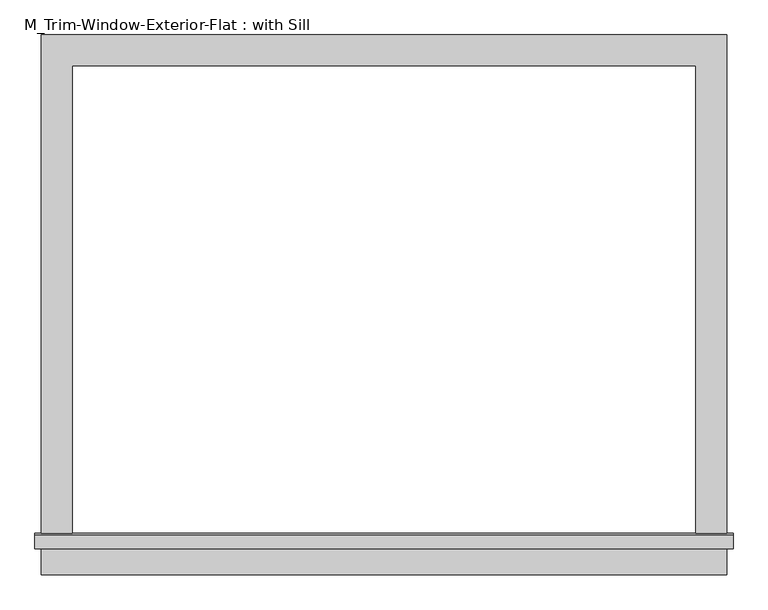
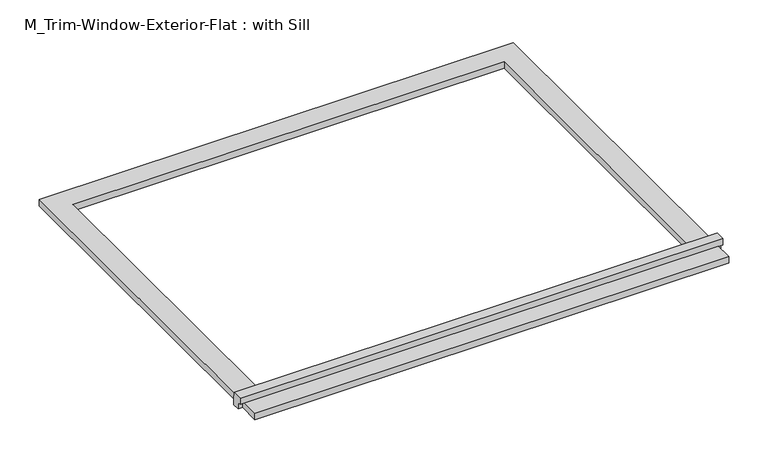
"""IFC4 building model written with IfcOpenShell, lengths in millimetres: proxy geometry, M_Trim-Window-Exterior-Flat : with Sill."""

from ifc_helpers import new_model, si_unit, frame, origin, origin_with_axes, place, context, project, spatial, polyline, outline, extrude, source, transform, mapped, element, save


def m_trim_window_exterior_flat_with_sill_6ae8fed8(model_context):
    return source(origin(), model_context, "Body", "SweptSolid", [
        extrude(outline(polyline([(669.6, -934.8323709), (669.6, -994.8323709), (-669.6, -994.8323709), (-669.6, -934.8323709), (669.6, -934.8323709)])), origin_with_axes(), (0.0, 0.0, 1.0), 19.05),
        extrude(outline(polyline([(-944.4, 38.1), (-916.8580645, 38.1), (-914.4, 19.05), (-914.4, 0.0), (-934.8323709, 0.0), (-934.8323709, 19.05), (-944.4, 19.05), (-944.4, 38.1)])), frame((-682.3, 0.0, 0.0), z_axis=(1.0, 0.0, 0.0), x_axis=(0.0, 1.0, 0.0)), (0.0, 0.0, 1.0), 1364.6),
        extrude(outline(polyline([(-669.6, 60.0), (669.6, 60.0), (669.6, -914.4), (609.6, -914.4), (609.6, 0.0), (-609.6, 0.0), (-609.6, -914.4), (-669.6, -914.4), (-669.6, 60.0)])), origin_with_axes(), (0.0, 0.0, 1.0), 19.05),
    ])


if __name__ == "__main__":
    model = new_model("IFC4")
    model_context = context("Model", 3, world=origin())
    ifc_project = project(units=[si_unit("LENGTHUNIT", "METRE", prefix="MILLI")], contexts=[model_context])
    site = spatial("IfcSite", under=ifc_project)
    building = spatial("IfcBuilding", under=site)
    placement = place(None, origin())
    m_trim_window_exterior_flat_with_sill_shape = m_trim_window_exterior_flat_with_sill_6ae8fed8(model_context)
    element("IfcBuildingElementProxy", 1, Name="M_Trim-Window-Exterior-Flat : with Sill", ObjectType="M_Trim-Window-Exterior-Flat : with Sill", at=placement, inside=building, context=model_context, shape_type="MappedRepresentation", body=[
        mapped(m_trim_window_exterior_flat_with_sill_shape, transform((0.0, 0.0, 0.0), x_axis=(1.0, 0.0, 0.0), y_axis=(0.0, 1.0, 0.0), z_axis=(0.0, 0.0, 1.0))),
    ])
    save(model, "model.ifc")

# Revit data of these elements
# Type "M_Trim-Window-Exterior-Flat : with Sill"
#   Trim Width = 0' - 2.3622"
#   Trim Thickness_Picture Frame = 0' - 1.1811"
#   Trim Thickness_with Sill = 0' - 0 3/4"
#   Sill Thickness = 0' - 1.1811"
#   Opening Width [instance default] = 1' - 11.62205"
#   Opening Height [instance default] = 2' - 11.43307"
#   Default Elevation = 3' - 11.24409"
#   Sill = yes
#   Picture Frame = no
#   Trim Material [instance default] = none
# Element 1 (IfcBuildingElementProxy, "M_Trim-Window-Exterior-Flat : with Sill")
#   Opening Width = 4' - 0"
#   Opening Height = 3' - 0"
#   Trim Material = Clad - White
#   Materials on its faces: "Clad - White"
# Materials
#   "Clad - White": class "Wood", colour RGB 242 242 238, transparency 0, Cost = 0
